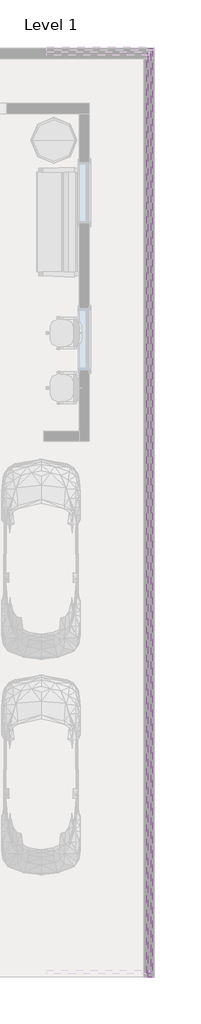
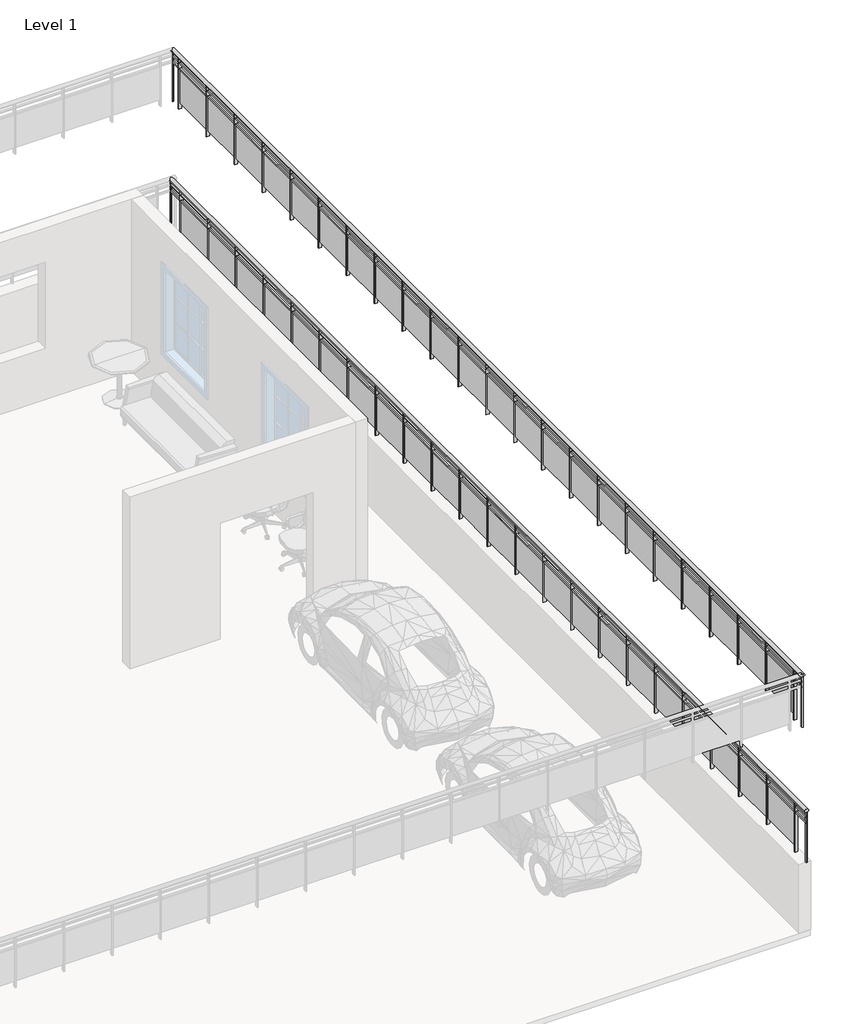
# One storey, part 4 of 6: 2 railings.
"""IFC4 building model written with IfcOpenShell, lengths in millimetres."""

from ifc_helpers import new_model, si_unit, point, frame, origin, place, context, project, spatial, polyline, ellipse_curve, trimmed, outline, extrude, element, save
from ifc_brep_helpers import plane_surface, extruded_surface, advanced_brep

model = new_model("IFC4")

# Units and contexts
model_context = context("Model", 3, world=origin())
ifc_project = project(units=[si_unit("LENGTHUNIT", "METRE", prefix="MILLI")], contexts=[model_context])

# Site, building, storey
site = spatial("IfcSite", under=ifc_project)
building = spatial("IfcBuilding", under=site)
storey = spatial("IfcBuildingStorey", under=building, Name="Level 1", Elevation=0.0)

# Railings
placement = place(None, origin())
element("IfcRailing", 1, ObjectType="Glass Panel - Bottom Fill", at=placement, inside=storey, context=model_context, shape_type="SolidModel", body=[
    advanced_brep(
    [(10487.1597674, -4490.3366944, 2133.6), (10563.3597674, -4490.3366944, 2133.6), (10487.1597674, 14000.8633056, 2133.6), (10563.3597674, 14000.8633056, 2133.6)],
    [
        (0, 1, ellipse_curve(frame((10525.2597674, -4490.3366944, 2133.6), z_axis=(0.0, -1.0, 0.0), x_axis=(1.0, 0.0, 0.0)), 38.1, 28.575)),
        (1, 0, ellipse_curve(frame((10525.2597674, -4490.3366944, 2133.6), z_axis=(0.0, -1.0, 0.0), x_axis=(1.0, 0.0, 0.0)), 38.1, 28.575)),
        (2, 3, ellipse_curve(frame((10525.2597674, 14000.8633056, 2133.6), z_axis=(0.0, 1.0, 0.0), x_axis=(1.0, 0.0, 0.0)), 38.1, 28.575)),
        (3, 2, ellipse_curve(frame((10525.2597674, 14000.8633056, 2133.6), z_axis=(0.0, 1.0, 0.0), x_axis=(1.0, 0.0, 0.0)), 38.1, 28.575)),
        (0, 2),
        (3, 1),
    ],
    [
        plane_surface(frame((10525.2597674, -4490.3366944, 2133.6), z_axis=(0.0, -1.0, 0.0), x_axis=(0.0, 0.0, 1.0))),
        plane_surface(frame((10525.2597674, 14000.8633056, 2133.6), z_axis=(0.0, 1.0, 0.0), x_axis=(0.0, 0.0, 1.0))),
        extruded_surface(trimmed(ellipse_curve(frame((10525.2597674, 14000.8633056, 2133.6), z_axis=(0.0, -1.0, 0.0), x_axis=(1.0, 0.0, 0.0)), 38.1, 28.575), [point((10487.1597674, 14000.8633056, 2133.6))], [point((10563.3597674, 14000.8633056, 2133.6))], True, "CARTESIAN"), (0.0, -18491.2, 0.0), 18491.2),
        extruded_surface(trimmed(ellipse_curve(frame((10525.2597674, 14000.8633056, 2133.6), z_axis=(0.0, -1.0, 0.0), x_axis=(1.0, 0.0, 0.0)), 38.1, 28.575), [point((10563.3597674, 14000.8633056, 2133.6))], [point((10487.1597674, 14000.8633056, 2133.6))], True, "CARTESIAN"), (0.0, -18491.2, 0.0), 18491.2),
    ],
    [
        (0, [[1, 2]]),
        (1, [[3, 4]]),
        (2, [[-1, 5, -4, 6]]),
        (3, [[-2, -6, -3, -5]]),
    ],
),
    extrude(outline(polyline([(10537.9597674, -4490.3366944), (10512.5597674, -4490.3366944), (10512.5597674, 14000.8633056), (10537.9597674, 14000.8633056), (10537.9597674, -4490.3366944)])), frame((0.0, 0.0, 2019.3), z_axis=(0.0, 0.0, 1.0), x_axis=(1.0, 0.0, 0.0)), (0.0, 0.0, 1.0), 25.4),
    extrude(outline(polyline([(10537.9597674, -4490.3366944), (10512.5597674, -4490.3366944), (10512.5597674, 14000.8633056), (10537.9597674, 14000.8633056), (10537.9597674, -4490.3366944)])), frame((0.0, 0.0, 1917.7), z_axis=(0.0, 0.0, 1.0), x_axis=(1.0, 0.0, 0.0)), (0.0, 0.0, 1.0), 25.4),
    extrude(outline(polyline([(10550.6597674, 13689.7133056), (10499.8597674, 13689.7133056), (10499.8597674, 13702.4133056), (10550.6597674, 13702.4133056), (10550.6597674, 13689.7133056)])), frame((0.0, 0.0, 1219.2), z_axis=(0.0, 0.0, 1.0), x_axis=(1.0, 0.0, 0.0)), (0.0, 0.0, 1.0), 885.6788223),
    extrude(outline(polyline([(10518.7246104, 12883.2633056), (10518.7246104, 13696.0633056), (10525.0746104, 13696.0633056), (10525.0746104, 12883.2633056), (10518.7246104, 12883.2633056)])), frame((0.0, 0.0, 1320.8), z_axis=(0.0, 0.0, 1.0), x_axis=(1.0, 0.0, 0.0)), (0.0, 0.0, 1.0), 596.9),
    extrude(outline(polyline([(10550.6597674, 12876.9133056), (10499.8597674, 12876.9133056), (10499.8597674, 12889.6133056), (10550.6597674, 12889.6133056), (10550.6597674, 12876.9133056)])), frame((0.0, 0.0, 1219.2), z_axis=(0.0, 0.0, 1.0), x_axis=(1.0, 0.0, 0.0)), (0.0, 0.0, 1.0), 885.6788223),
    extrude(outline(polyline([(10518.7246104, 12070.4633056), (10518.7246104, 12883.2633056), (10525.0746104, 12883.2633056), (10525.0746104, 12070.4633056), (10518.7246104, 12070.4633056)])), frame((0.0, 0.0, 1320.8), z_axis=(0.0, 0.0, 1.0), x_axis=(1.0, 0.0, 0.0)), (0.0, 0.0, 1.0), 596.9),
    extrude(outline(polyline([(10550.6597674, 12064.1133056), (10499.8597674, 12064.1133056), (10499.8597674, 12076.8133056), (10550.6597674, 12076.8133056), (10550.6597674, 12064.1133056)])), frame((0.0, 0.0, 1219.2), z_axis=(0.0, 0.0, 1.0), x_axis=(1.0, 0.0, 0.0)), (0.0, 0.0, 1.0), 885.6788223),
    extrude(outline(polyline([(10518.7246104, 11257.6633056), (10518.7246104, 12070.4633056), (10525.0746104, 12070.4633056), (10525.0746104, 11257.6633056), (10518.7246104, 11257.6633056)])), frame((0.0, 0.0, 1320.8), z_axis=(0.0, 0.0, 1.0), x_axis=(1.0, 0.0, 0.0)), (0.0, 0.0, 1.0), 596.9),
    extrude(outline(polyline([(10550.6597674, 11251.3133056), (10499.8597674, 11251.3133056), (10499.8597674, 11264.0133056), (10550.6597674, 11264.0133056), (10550.6597674, 11251.3133056)])), frame((0.0, 0.0, 1219.2), z_axis=(0.0, 0.0, 1.0), x_axis=(1.0, 0.0, 0.0)), (0.0, 0.0, 1.0), 885.6788223),
    extrude(outline(polyline([(10518.7246104, 10444.8633056), (10518.7246104, 11257.6633056), (10525.0746104, 11257.6633056), (10525.0746104, 10444.8633056), (10518.7246104, 10444.8633056)])), frame((0.0, 0.0, 1320.8), z_axis=(0.0, 0.0, 1.0), x_axis=(1.0, 0.0, 0.0)), (0.0, 0.0, 1.0), 596.9),
    extrude(outline(polyline([(10550.6597674, 10438.5133056), (10499.8597674, 10438.5133056), (10499.8597674, 10451.2133056), (10550.6597674, 10451.2133056), (10550.6597674, 10438.5133056)])), frame((0.0, 0.0, 1219.2), z_axis=(0.0, 0.0, 1.0), x_axis=(1.0, 0.0, 0.0)), (0.0, 0.0, 1.0), 885.6788223),
    extrude(outline(polyline([(10518.7246104, 9632.0633056), (10518.7246104, 10444.8633056), (10525.0746104, 10444.8633056), (10525.0746104, 9632.0633056), (10518.7246104, 9632.0633056)])), frame((0.0, 0.0, 1320.8), z_axis=(0.0, 0.0, 1.0), x_axis=(1.0, 0.0, 0.0)), (0.0, 0.0, 1.0), 596.9),
    extrude(outline(polyline([(10550.6597674, 9625.7133056), (10499.8597674, 9625.7133056), (10499.8597674, 9638.4133056), (10550.6597674, 9638.4133056), (10550.6597674, 9625.7133056)])), frame((0.0, 0.0, 1219.2), z_axis=(0.0, 0.0, 1.0), x_axis=(1.0, 0.0, 0.0)), (0.0, 0.0, 1.0), 885.6788223),
    extrude(outline(polyline([(10518.7246104, 8819.2633056), (10518.7246104, 9632.0633056), (10525.0746104, 9632.0633056), (10525.0746104, 8819.2633056), (10518.7246104, 8819.2633056)])), frame((0.0, 0.0, 1320.8), z_axis=(0.0, 0.0, 1.0), x_axis=(1.0, 0.0, 0.0)), (0.0, 0.0, 1.0), 596.9),
    extrude(outline(polyline([(10550.6597674, 8812.9133056), (10499.8597674, 8812.9133056), (10499.8597674, 8825.6133056), (10550.6597674, 8825.6133056), (10550.6597674, 8812.9133056)])), frame((0.0, 0.0, 1219.2), z_axis=(0.0, 0.0, 1.0), x_axis=(1.0, 0.0, 0.0)), (0.0, 0.0, 1.0), 885.6788223),
    extrude(outline(polyline([(10518.7246104, 8006.4633056), (10518.7246104, 8819.2633056), (10525.0746104, 8819.2633056), (10525.0746104, 8006.4633056), (10518.7246104, 8006.4633056)])), frame((0.0, 0.0, 1320.8), z_axis=(0.0, 0.0, 1.0), x_axis=(1.0, 0.0, 0.0)), (0.0, 0.0, 1.0), 596.9),
    extrude(outline(polyline([(10550.6597674, 8000.1133056), (10499.8597674, 8000.1133056), (10499.8597674, 8012.8133056), (10550.6597674, 8012.8133056), (10550.6597674, 8000.1133056)])), frame((0.0, 0.0, 1219.2), z_axis=(0.0, 0.0, 1.0), x_axis=(1.0, 0.0, 0.0)), (0.0, 0.0, 1.0), 885.6788223),
    extrude(outline(polyline([(10518.7246104, 7193.6633056), (10518.7246104, 8006.4633056), (10525.0746104, 8006.4633056), (10525.0746104, 7193.6633056), (10518.7246104, 7193.6633056)])), frame((0.0, 0.0, 1320.8), z_axis=(0.0, 0.0, 1.0), x_axis=(1.0, 0.0, 0.0)), (0.0, 0.0, 1.0), 596.9),
    extrude(outline(polyline([(10550.6597674, 7187.3133056), (10499.8597674, 7187.3133056), (10499.8597674, 7200.0133056), (10550.6597674, 7200.0133056), (10550.6597674, 7187.3133056)])), frame((0.0, 0.0, 1219.2), z_axis=(0.0, 0.0, 1.0), x_axis=(1.0, 0.0, 0.0)), (0.0, 0.0, 1.0), 885.6788223),
    extrude(outline(polyline([(10518.7246104, 6380.8633056), (10518.7246104, 7193.6633056), (10525.0746104, 7193.6633056), (10525.0746104, 6380.8633056), (10518.7246104, 6380.8633056)])), frame((0.0, 0.0, 1320.8), z_axis=(0.0, 0.0, 1.0), x_axis=(1.0, 0.0, 0.0)), (0.0, 0.0, 1.0), 596.9),
    extrude(outline(polyline([(10550.6597674, 6374.5133056), (10499.8597674, 6374.5133056), (10499.8597674, 6387.2133056), (10550.6597674, 6387.2133056), (10550.6597674, 6374.5133056)])), frame((0.0, 0.0, 1219.2), z_axis=(0.0, 0.0, 1.0), x_axis=(1.0, 0.0, 0.0)), (0.0, 0.0, 1.0), 885.6788223),
    extrude(outline(polyline([(10518.7246104, 5568.0633056), (10518.7246104, 6380.8633056), (10525.0746104, 6380.8633056), (10525.0746104, 5568.0633056), (10518.7246104, 5568.0633056)])), frame((0.0, 0.0, 1320.8), z_axis=(0.0, 0.0, 1.0), x_axis=(1.0, 0.0, 0.0)), (0.0, 0.0, 1.0), 596.9),
    extrude(outline(polyline([(10550.6597674, 5561.7133056), (10499.8597674, 5561.7133056), (10499.8597674, 5574.4133056), (10550.6597674, 5574.4133056), (10550.6597674, 5561.7133056)])), frame((0.0, 0.0, 1219.2), z_axis=(0.0, 0.0, 1.0), x_axis=(1.0, 0.0, 0.0)), (0.0, 0.0, 1.0), 885.6788223),
    extrude(outline(polyline([(10518.7246104, 4755.2633056), (10518.7246104, 5568.0633056), (10525.0746104, 5568.0633056), (10525.0746104, 4755.2633056), (10518.7246104, 4755.2633056)])), frame((0.0, 0.0, 1320.8), z_axis=(0.0, 0.0, 1.0), x_axis=(1.0, 0.0, 0.0)), (0.0, 0.0, 1.0), 596.9),
    extrude(outline(polyline([(10550.6597674, 4748.9133056), (10499.8597674, 4748.9133056), (10499.8597674, 4761.6133056), (10550.6597674, 4761.6133056), (10550.6597674, 4748.9133056)])), frame((0.0, 0.0, 1219.2), z_axis=(0.0, 0.0, 1.0), x_axis=(1.0, 0.0, 0.0)), (0.0, 0.0, 1.0), 885.6788223),
    extrude(outline(polyline([(10518.7246104, 3942.4633056), (10518.7246104, 4755.2633056), (10525.0746104, 4755.2633056), (10525.0746104, 3942.4633056), (10518.7246104, 3942.4633056)])), frame((0.0, 0.0, 1320.8), z_axis=(0.0, 0.0, 1.0), x_axis=(1.0, 0.0, 0.0)), (0.0, 0.0, 1.0), 596.9),
    extrude(outline(polyline([(10550.6597674, 3936.1133056), (10499.8597674, 3936.1133056), (10499.8597674, 3948.8133056), (10550.6597674, 3948.8133056), (10550.6597674, 3936.1133056)])), frame((0.0, 0.0, 1219.2), z_axis=(0.0, 0.0, 1.0), x_axis=(1.0, 0.0, 0.0)), (0.0, 0.0, 1.0), 885.6788223),
    extrude(outline(polyline([(10518.7246104, 3129.6633056), (10518.7246104, 3942.4633056), (10525.0746104, 3942.4633056), (10525.0746104, 3129.6633056), (10518.7246104, 3129.6633056)])), frame((0.0, 0.0, 1320.8), z_axis=(0.0, 0.0, 1.0), x_axis=(1.0, 0.0, 0.0)), (0.0, 0.0, 1.0), 596.9),
    extrude(outline(polyline([(10550.6597674, 3123.3133056), (10499.8597674, 3123.3133056), (10499.8597674, 3136.0133056), (10550.6597674, 3136.0133056), (10550.6597674, 3123.3133056)])), frame((0.0, 0.0, 1219.2), z_axis=(0.0, 0.0, 1.0), x_axis=(1.0, 0.0, 0.0)), (0.0, 0.0, 1.0), 885.6788223),
    extrude(outline(polyline([(10518.7246104, 2316.8633056), (10518.7246104, 3129.6633056), (10525.0746104, 3129.6633056), (10525.0746104, 2316.8633056), (10518.7246104, 2316.8633056)])), frame((0.0, 0.0, 1320.8), z_axis=(0.0, 0.0, 1.0), x_axis=(1.0, 0.0, 0.0)), (0.0, 0.0, 1.0), 596.9),
    extrude(outline(polyline([(10550.6597674, 2310.5133056), (10499.8597674, 2310.5133056), (10499.8597674, 2323.2133056), (10550.6597674, 2323.2133056), (10550.6597674, 2310.5133056)])), frame((0.0, 0.0, 1219.2), z_axis=(0.0, 0.0, 1.0), x_axis=(1.0, 0.0, 0.0)), (0.0, 0.0, 1.0), 885.6788223),
    extrude(outline(polyline([(10518.7246104, 1504.0633056), (10518.7246104, 2316.8633056), (10525.0746104, 2316.8633056), (10525.0746104, 1504.0633056), (10518.7246104, 1504.0633056)])), frame((0.0, 0.0, 1320.8), z_axis=(0.0, 0.0, 1.0), x_axis=(1.0, 0.0, 0.0)), (0.0, 0.0, 1.0), 596.9),
    extrude(outline(polyline([(10550.6597674, 1497.7133056), (10499.8597674, 1497.7133056), (10499.8597674, 1510.4133056), (10550.6597674, 1510.4133056), (10550.6597674, 1497.7133056)])), frame((0.0, 0.0, 1219.2), z_axis=(0.0, 0.0, 1.0), x_axis=(1.0, 0.0, 0.0)), (0.0, 0.0, 1.0), 885.6788223),
    extrude(outline(polyline([(10518.7246104, 691.2633056), (10518.7246104, 1504.0633056), (10525.0746104, 1504.0633056), (10525.0746104, 691.2633056), (10518.7246104, 691.2633056)])), frame((0.0, 0.0, 1320.8), z_axis=(0.0, 0.0, 1.0), x_axis=(1.0, 0.0, 0.0)), (0.0, 0.0, 1.0), 596.9),
    extrude(outline(polyline([(10550.6597674, 684.9133056), (10499.8597674, 684.9133056), (10499.8597674, 697.6133056), (10550.6597674, 697.6133056), (10550.6597674, 684.9133056)])), frame((0.0, 0.0, 1219.2), z_axis=(0.0, 0.0, 1.0), x_axis=(1.0, 0.0, 0.0)), (0.0, 0.0, 1.0), 885.6788223),
    extrude(outline(polyline([(10518.7246104, -121.5366944), (10518.7246104, 691.2633056), (10525.0746104, 691.2633056), (10525.0746104, -121.5366944), (10518.7246104, -121.5366944)])), frame((0.0, 0.0, 1320.8), z_axis=(0.0, 0.0, 1.0), x_axis=(1.0, 0.0, 0.0)), (0.0, 0.0, 1.0), 596.9),
    extrude(outline(polyline([(10550.6597674, -127.8866944), (10499.8597674, -127.8866944), (10499.8597674, -115.1866944), (10550.6597674, -115.1866944), (10550.6597674, -127.8866944)])), frame((0.0, 0.0, 1219.2), z_axis=(0.0, 0.0, 1.0), x_axis=(1.0, 0.0, 0.0)), (0.0, 0.0, 1.0), 885.6788223),
    extrude(outline(polyline([(10518.7246104, -934.3366944), (10518.7246104, -121.5366944), (10525.0746104, -121.5366944), (10525.0746104, -934.3366944), (10518.7246104, -934.3366944)])), frame((0.0, 0.0, 1320.8), z_axis=(0.0, 0.0, 1.0), x_axis=(1.0, 0.0, 0.0)), (0.0, 0.0, 1.0), 596.9),
    extrude(outline(polyline([(10550.6597674, -940.6866944), (10499.8597674, -940.6866944), (10499.8597674, -927.9866944), (10550.6597674, -927.9866944), (10550.6597674, -940.6866944)])), frame((0.0, 0.0, 1219.2), z_axis=(0.0, 0.0, 1.0), x_axis=(1.0, 0.0, 0.0)), (0.0, 0.0, 1.0), 885.6788223),
    extrude(outline(polyline([(10518.7246104, -1747.1366944), (10518.7246104, -934.3366944), (10525.0746104, -934.3366944), (10525.0746104, -1747.1366944), (10518.7246104, -1747.1366944)])), frame((0.0, 0.0, 1320.8), z_axis=(0.0, 0.0, 1.0), x_axis=(1.0, 0.0, 0.0)), (0.0, 0.0, 1.0), 596.9),
    extrude(outline(polyline([(10550.6597674, -1753.4866944), (10499.8597674, -1753.4866944), (10499.8597674, -1740.7866944), (10550.6597674, -1740.7866944), (10550.6597674, -1753.4866944)])), frame((0.0, 0.0, 1219.2), z_axis=(0.0, 0.0, 1.0), x_axis=(1.0, 0.0, 0.0)), (0.0, 0.0, 1.0), 885.6788223),
    extrude(outline(polyline([(10518.7246104, -2559.9366944), (10518.7246104, -1747.1366944), (10525.0746104, -1747.1366944), (10525.0746104, -2559.9366944), (10518.7246104, -2559.9366944)])), frame((0.0, 0.0, 1320.8), z_axis=(0.0, 0.0, 1.0), x_axis=(1.0, 0.0, 0.0)), (0.0, 0.0, 1.0), 596.9),
    extrude(outline(polyline([(10550.6597674, -2566.2866944), (10499.8597674, -2566.2866944), (10499.8597674, -2553.5866944), (10550.6597674, -2553.5866944), (10550.6597674, -2566.2866944)])), frame((0.0, 0.0, 1219.2), z_axis=(0.0, 0.0, 1.0), x_axis=(1.0, 0.0, 0.0)), (0.0, 0.0, 1.0), 885.6788223),
    extrude(outline(polyline([(10518.7246104, -3372.7366944), (10518.7246104, -2559.9366944), (10525.0746104, -2559.9366944), (10525.0746104, -3372.7366944), (10518.7246104, -3372.7366944)])), frame((0.0, 0.0, 1320.8), z_axis=(0.0, 0.0, 1.0), x_axis=(1.0, 0.0, 0.0)), (0.0, 0.0, 1.0), 596.9),
    extrude(outline(polyline([(10550.6597674, -3379.0866944), (10499.8597674, -3379.0866944), (10499.8597674, -3366.3866944), (10550.6597674, -3366.3866944), (10550.6597674, -3379.0866944)])), frame((0.0, 0.0, 1219.2), z_axis=(0.0, 0.0, 1.0), x_axis=(1.0, 0.0, 0.0)), (0.0, 0.0, 1.0), 885.6788223),
    extrude(outline(polyline([(10518.7246104, -4185.5366944), (10518.7246104, -3372.7366944), (10525.0746104, -3372.7366944), (10525.0746104, -4185.5366944), (10518.7246104, -4185.5366944)])), frame((0.0, 0.0, 1320.8), z_axis=(0.0, 0.0, 1.0), x_axis=(1.0, 0.0, 0.0)), (0.0, 0.0, 1.0), 596.9),
    extrude(outline(polyline([(10550.6597674, -4191.8866944), (10499.8597674, -4191.8866944), (10499.8597674, -4179.1866944), (10550.6597674, -4179.1866944), (10550.6597674, -4191.8866944)])), frame((0.0, 0.0, 1219.2), z_axis=(0.0, 0.0, 1.0), x_axis=(1.0, 0.0, 0.0)), (0.0, 0.0, 1.0), 885.6788223),
    extrude(outline(polyline([(10534.7847674, 13988.1633056), (10515.7347674, 13988.1633056), (10515.7347674, 14007.2133056), (10534.7847674, 14007.2133056), (10534.7847674, 13988.1633056)])), frame((0.0, 0.0, 1219.2), z_axis=(0.0, 0.0, 1.0), x_axis=(1.0, 0.0, 0.0)), (0.0, 0.0, 1.0), 885.6788223),
    extrude(outline(polyline([(10534.7847674, -4496.6866944), (10515.7347674, -4496.6866944), (10515.7347674, -4477.6366944), (10534.7847674, -4477.6366944), (10534.7847674, -4496.6866944)])), frame((0.0, 0.0, 1219.2), z_axis=(0.0, 0.0, 1.0), x_axis=(1.0, 0.0, 0.0)), (0.0, 0.0, 1.0), 885.6788223),
])
element("IfcRailing", 2, ObjectType="Glass Panel - Bottom Fill", at=placement, inside=storey, context=model_context, shape_type="SolidModel", body=[
    advanced_brep(
    [(10461.7597674, -4414.1366944, 4495.8), (10537.9597674, -4414.1366944, 4495.8), (10461.7597674, 13899.2633056, 4495.8), (10537.9597674, 13899.2633056, 4495.8)],
    [
        (0, 1, ellipse_curve(frame((10499.8597674, -4414.1366944, 4495.8), z_axis=(0.0, -1.0, 0.0), x_axis=(1.0, 0.0, 0.0)), 38.1, 28.575)),
        (1, 0, ellipse_curve(frame((10499.8597674, -4414.1366944, 4495.8), z_axis=(0.0, -1.0, 0.0), x_axis=(1.0, 0.0, 0.0)), 38.1, 28.575)),
        (2, 3, ellipse_curve(frame((10499.8597674, 13899.2633056, 4495.8), z_axis=(0.0, 1.0, 0.0), x_axis=(1.0, 0.0, 0.0)), 38.1, 28.575)),
        (3, 2, ellipse_curve(frame((10499.8597674, 13899.2633056, 4495.8), z_axis=(0.0, 1.0, 0.0), x_axis=(1.0, 0.0, 0.0)), 38.1, 28.575)),
        (0, 2),
        (3, 1),
    ],
    [
        plane_surface(frame((10499.8597674, -4414.1366944, 4495.8), z_axis=(0.0, -1.0, 0.0), x_axis=(0.0, 0.0, 1.0))),
        plane_surface(frame((10499.8597674, 13899.2633056, 4495.8), z_axis=(0.0, 1.0, 0.0), x_axis=(0.0, 0.0, 1.0))),
        extruded_surface(trimmed(ellipse_curve(frame((10499.8597674, 13899.2633056, 4495.8), z_axis=(0.0, -1.0, 0.0), x_axis=(1.0, 0.0, 0.0)), 38.1, 28.575), [point((10461.7597674, 13899.2633056, 4495.8))], [point((10537.9597674, 13899.2633056, 4495.8))], True, "CARTESIAN"), (0.0, -18313.4, 0.0), 18313.4),
        extruded_surface(trimmed(ellipse_curve(frame((10499.8597674, 13899.2633056, 4495.8), z_axis=(0.0, -1.0, 0.0), x_axis=(1.0, 0.0, 0.0)), 38.1, 28.575), [point((10537.9597674, 13899.2633056, 4495.8))], [point((10461.7597674, 13899.2633056, 4495.8))], True, "CARTESIAN"), (0.0, -18313.4, 0.0), 18313.4),
    ],
    [
        (0, [[1, 2]]),
        (1, [[3, 4]]),
        (2, [[-1, 5, -4, 6]]),
        (3, [[-2, -6, -3, -5]]),
    ],
),
    extrude(outline(polyline([(10512.5597674, -4414.1366944), (10487.1597674, -4414.1366944), (10487.1597674, 13899.2633056), (10512.5597674, 13899.2633056), (10512.5597674, -4414.1366944)])), frame((0.0, 0.0, 4381.5), z_axis=(0.0, 0.0, 1.0), x_axis=(1.0, 0.0, 0.0)), (0.0, 0.0, 1.0), 25.4),
    extrude(outline(polyline([(10512.5597674, -4414.1366944), (10487.1597674, -4414.1366944), (10487.1597674, 13899.2633056), (10512.5597674, 13899.2633056), (10512.5597674, -4414.1366944)])), frame((0.0, 0.0, 4279.9), z_axis=(0.0, 0.0, 1.0), x_axis=(1.0, 0.0, 0.0)), (0.0, 0.0, 1.0), 25.4),
    extrude(outline(polyline([(10525.2597674, 13677.0133056), (10474.4597674, 13677.0133056), (10474.4597674, 13689.7133056), (10525.2597674, 13689.7133056), (10525.2597674, 13677.0133056)])), frame((0.0, 0.0, 3581.4), z_axis=(0.0, 0.0, 1.0), x_axis=(1.0, 0.0, 0.0)), (0.0, 0.0, 1.0), 885.6788223),
    extrude(outline(polyline([(10493.3246104, 12870.5633056), (10493.3246104, 13683.3633056), (10499.6746104, 13683.3633056), (10499.6746104, 12870.5633056), (10493.3246104, 12870.5633056)])), frame((0.0, 0.0, 3683.0), z_axis=(0.0, 0.0, 1.0), x_axis=(1.0, 0.0, 0.0)), (0.0, 0.0, 1.0), 596.9),
    extrude(outline(polyline([(10525.2597674, 12864.2133056), (10474.4597674, 12864.2133056), (10474.4597674, 12876.9133056), (10525.2597674, 12876.9133056), (10525.2597674, 12864.2133056)])), frame((0.0, 0.0, 3581.4), z_axis=(0.0, 0.0, 1.0), x_axis=(1.0, 0.0, 0.0)), (0.0, 0.0, 1.0), 885.6788223),
    extrude(outline(polyline([(10493.3246104, 12057.7633056), (10493.3246104, 12870.5633056), (10499.6746104, 12870.5633056), (10499.6746104, 12057.7633056), (10493.3246104, 12057.7633056)])), frame((0.0, 0.0, 3683.0), z_axis=(0.0, 0.0, 1.0), x_axis=(1.0, 0.0, 0.0)), (0.0, 0.0, 1.0), 596.9),
    extrude(outline(polyline([(10525.2597674, 12051.4133056), (10474.4597674, 12051.4133056), (10474.4597674, 12064.1133056), (10525.2597674, 12064.1133056), (10525.2597674, 12051.4133056)])), frame((0.0, 0.0, 3581.4), z_axis=(0.0, 0.0, 1.0), x_axis=(1.0, 0.0, 0.0)), (0.0, 0.0, 1.0), 885.6788223),
    extrude(outline(polyline([(10493.3246104, 11244.9633056), (10493.3246104, 12057.7633056), (10499.6746104, 12057.7633056), (10499.6746104, 11244.9633056), (10493.3246104, 11244.9633056)])), frame((0.0, 0.0, 3683.0), z_axis=(0.0, 0.0, 1.0), x_axis=(1.0, 0.0, 0.0)), (0.0, 0.0, 1.0), 596.9),
    extrude(outline(polyline([(10525.2597674, 11238.6133056), (10474.4597674, 11238.6133056), (10474.4597674, 11251.3133056), (10525.2597674, 11251.3133056), (10525.2597674, 11238.6133056)])), frame((0.0, 0.0, 3581.4), z_axis=(0.0, 0.0, 1.0), x_axis=(1.0, 0.0, 0.0)), (0.0, 0.0, 1.0), 885.6788223),
    extrude(outline(polyline([(10493.3246104, 10432.1633056), (10493.3246104, 11244.9633056), (10499.6746104, 11244.9633056), (10499.6746104, 10432.1633056), (10493.3246104, 10432.1633056)])), frame((0.0, 0.0, 3683.0), z_axis=(0.0, 0.0, 1.0), x_axis=(1.0, 0.0, 0.0)), (0.0, 0.0, 1.0), 596.9),
    extrude(outline(polyline([(10525.2597674, 10425.8133056), (10474.4597674, 10425.8133056), (10474.4597674, 10438.5133056), (10525.2597674, 10438.5133056), (10525.2597674, 10425.8133056)])), frame((0.0, 0.0, 3581.4), z_axis=(0.0, 0.0, 1.0), x_axis=(1.0, 0.0, 0.0)), (0.0, 0.0, 1.0), 885.6788223),
    extrude(outline(polyline([(10493.3246104, 9619.3633056), (10493.3246104, 10432.1633056), (10499.6746104, 10432.1633056), (10499.6746104, 9619.3633056), (10493.3246104, 9619.3633056)])), frame((0.0, 0.0, 3683.0), z_axis=(0.0, 0.0, 1.0), x_axis=(1.0, 0.0, 0.0)), (0.0, 0.0, 1.0), 596.9),
    extrude(outline(polyline([(10525.2597674, 9613.0133056), (10474.4597674, 9613.0133056), (10474.4597674, 9625.7133056), (10525.2597674, 9625.7133056), (10525.2597674, 9613.0133056)])), frame((0.0, 0.0, 3581.4), z_axis=(0.0, 0.0, 1.0), x_axis=(1.0, 0.0, 0.0)), (0.0, 0.0, 1.0), 885.6788223),
    extrude(outline(polyline([(10493.3246104, 8806.5633056), (10493.3246104, 9619.3633056), (10499.6746104, 9619.3633056), (10499.6746104, 8806.5633056), (10493.3246104, 8806.5633056)])), frame((0.0, 0.0, 3683.0), z_axis=(0.0, 0.0, 1.0), x_axis=(1.0, 0.0, 0.0)), (0.0, 0.0, 1.0), 596.9),
    extrude(outline(polyline([(10525.2597674, 8800.2133056), (10474.4597674, 8800.2133056), (10474.4597674, 8812.9133056), (10525.2597674, 8812.9133056), (10525.2597674, 8800.2133056)])), frame((0.0, 0.0, 3581.4), z_axis=(0.0, 0.0, 1.0), x_axis=(1.0, 0.0, 0.0)), (0.0, 0.0, 1.0), 885.6788223),
    extrude(outline(polyline([(10493.3246104, 7993.7633056), (10493.3246104, 8806.5633056), (10499.6746104, 8806.5633056), (10499.6746104, 7993.7633056), (10493.3246104, 7993.7633056)])), frame((0.0, 0.0, 3683.0), z_axis=(0.0, 0.0, 1.0), x_axis=(1.0, 0.0, 0.0)), (0.0, 0.0, 1.0), 596.9),
    extrude(outline(polyline([(10525.2597674, 7987.4133056), (10474.4597674, 7987.4133056), (10474.4597674, 8000.1133056), (10525.2597674, 8000.1133056), (10525.2597674, 7987.4133056)])), frame((0.0, 0.0, 3581.4), z_axis=(0.0, 0.0, 1.0), x_axis=(1.0, 0.0, 0.0)), (0.0, 0.0, 1.0), 885.6788223),
    extrude(outline(polyline([(10493.3246104, 7180.9633056), (10493.3246104, 7993.7633056), (10499.6746104, 7993.7633056), (10499.6746104, 7180.9633056), (10493.3246104, 7180.9633056)])), frame((0.0, 0.0, 3683.0), z_axis=(0.0, 0.0, 1.0), x_axis=(1.0, 0.0, 0.0)), (0.0, 0.0, 1.0), 596.9),
    extrude(outline(polyline([(10525.2597674, 7174.6133056), (10474.4597674, 7174.6133056), (10474.4597674, 7187.3133056), (10525.2597674, 7187.3133056), (10525.2597674, 7174.6133056)])), frame((0.0, 0.0, 3581.4), z_axis=(0.0, 0.0, 1.0), x_axis=(1.0, 0.0, 0.0)), (0.0, 0.0, 1.0), 885.6788223),
    extrude(outline(polyline([(10493.3246104, 6368.1633056), (10493.3246104, 7180.9633056), (10499.6746104, 7180.9633056), (10499.6746104, 6368.1633056), (10493.3246104, 6368.1633056)])), frame((0.0, 0.0, 3683.0), z_axis=(0.0, 0.0, 1.0), x_axis=(1.0, 0.0, 0.0)), (0.0, 0.0, 1.0), 596.9),
    extrude(outline(polyline([(10525.2597674, 6361.8133056), (10474.4597674, 6361.8133056), (10474.4597674, 6374.5133056), (10525.2597674, 6374.5133056), (10525.2597674, 6361.8133056)])), frame((0.0, 0.0, 3581.4), z_axis=(0.0, 0.0, 1.0), x_axis=(1.0, 0.0, 0.0)), (0.0, 0.0, 1.0), 885.6788223),
    extrude(outline(polyline([(10493.3246104, 5555.3633056), (10493.3246104, 6368.1633056), (10499.6746104, 6368.1633056), (10499.6746104, 5555.3633056), (10493.3246104, 5555.3633056)])), frame((0.0, 0.0, 3683.0), z_axis=(0.0, 0.0, 1.0), x_axis=(1.0, 0.0, 0.0)), (0.0, 0.0, 1.0), 596.9),
    extrude(outline(polyline([(10525.2597674, 5549.0133056), (10474.4597674, 5549.0133056), (10474.4597674, 5561.7133056), (10525.2597674, 5561.7133056), (10525.2597674, 5549.0133056)])), frame((0.0, 0.0, 3581.4), z_axis=(0.0, 0.0, 1.0), x_axis=(1.0, 0.0, 0.0)), (0.0, 0.0, 1.0), 885.6788223),
    extrude(outline(polyline([(10493.3246104, 4742.5633056), (10493.3246104, 5555.3633056), (10499.6746104, 5555.3633056), (10499.6746104, 4742.5633056), (10493.3246104, 4742.5633056)])), frame((0.0, 0.0, 3683.0), z_axis=(0.0, 0.0, 1.0), x_axis=(1.0, 0.0, 0.0)), (0.0, 0.0, 1.0), 596.9),
    extrude(outline(polyline([(10525.2597674, 4736.2133056), (10474.4597674, 4736.2133056), (10474.4597674, 4748.9133056), (10525.2597674, 4748.9133056), (10525.2597674, 4736.2133056)])), frame((0.0, 0.0, 3581.4), z_axis=(0.0, 0.0, 1.0), x_axis=(1.0, 0.0, 0.0)), (0.0, 0.0, 1.0), 885.6788223),
    extrude(outline(polyline([(10493.3246104, 3929.7633056), (10493.3246104, 4742.5633056), (10499.6746104, 4742.5633056), (10499.6746104, 3929.7633056), (10493.3246104, 3929.7633056)])), frame((0.0, 0.0, 3683.0), z_axis=(0.0, 0.0, 1.0), x_axis=(1.0, 0.0, 0.0)), (0.0, 0.0, 1.0), 596.9),
    extrude(outline(polyline([(10525.2597674, 3923.4133056), (10474.4597674, 3923.4133056), (10474.4597674, 3936.1133056), (10525.2597674, 3936.1133056), (10525.2597674, 3923.4133056)])), frame((0.0, 0.0, 3581.4), z_axis=(0.0, 0.0, 1.0), x_axis=(1.0, 0.0, 0.0)), (0.0, 0.0, 1.0), 885.6788223),
    extrude(outline(polyline([(10493.3246104, 3116.9633056), (10493.3246104, 3929.7633056), (10499.6746104, 3929.7633056), (10499.6746104, 3116.9633056), (10493.3246104, 3116.9633056)])), frame((0.0, 0.0, 3683.0), z_axis=(0.0, 0.0, 1.0), x_axis=(1.0, 0.0, 0.0)), (0.0, 0.0, 1.0), 596.9),
    extrude(outline(polyline([(10525.2597674, 3110.6133056), (10474.4597674, 3110.6133056), (10474.4597674, 3123.3133056), (10525.2597674, 3123.3133056), (10525.2597674, 3110.6133056)])), frame((0.0, 0.0, 3581.4), z_axis=(0.0, 0.0, 1.0), x_axis=(1.0, 0.0, 0.0)), (0.0, 0.0, 1.0), 885.6788223),
    extrude(outline(polyline([(10493.3246104, 2304.1633056), (10493.3246104, 3116.9633056), (10499.6746104, 3116.9633056), (10499.6746104, 2304.1633056), (10493.3246104, 2304.1633056)])), frame((0.0, 0.0, 3683.0), z_axis=(0.0, 0.0, 1.0), x_axis=(1.0, 0.0, 0.0)), (0.0, 0.0, 1.0), 596.9),
    extrude(outline(polyline([(10525.2597674, 2297.8133056), (10474.4597674, 2297.8133056), (10474.4597674, 2310.5133056), (10525.2597674, 2310.5133056), (10525.2597674, 2297.8133056)])), frame((0.0, 0.0, 3581.4), z_axis=(0.0, 0.0, 1.0), x_axis=(1.0, 0.0, 0.0)), (0.0, 0.0, 1.0), 885.6788223),
    extrude(outline(polyline([(10493.3246104, 1491.3633056), (10493.3246104, 2304.1633056), (10499.6746104, 2304.1633056), (10499.6746104, 1491.3633056), (10493.3246104, 1491.3633056)])), frame((0.0, 0.0, 3683.0), z_axis=(0.0, 0.0, 1.0), x_axis=(1.0, 0.0, 0.0)), (0.0, 0.0, 1.0), 596.9),
    extrude(outline(polyline([(10525.2597674, 1485.0133056), (10474.4597674, 1485.0133056), (10474.4597674, 1497.7133056), (10525.2597674, 1497.7133056), (10525.2597674, 1485.0133056)])), frame((0.0, 0.0, 3581.4), z_axis=(0.0, 0.0, 1.0), x_axis=(1.0, 0.0, 0.0)), (0.0, 0.0, 1.0), 885.6788223),
    extrude(outline(polyline([(10493.3246104, 678.5633056), (10493.3246104, 1491.3633056), (10499.6746104, 1491.3633056), (10499.6746104, 678.5633056), (10493.3246104, 678.5633056)])), frame((0.0, 0.0, 3683.0), z_axis=(0.0, 0.0, 1.0), x_axis=(1.0, 0.0, 0.0)), (0.0, 0.0, 1.0), 596.9),
    extrude(outline(polyline([(10525.2597674, 672.2133056), (10474.4597674, 672.2133056), (10474.4597674, 684.9133056), (10525.2597674, 684.9133056), (10525.2597674, 672.2133056)])), frame((0.0, 0.0, 3581.4), z_axis=(0.0, 0.0, 1.0), x_axis=(1.0, 0.0, 0.0)), (0.0, 0.0, 1.0), 885.6788223),
    extrude(outline(polyline([(10493.3246104, -134.2366944), (10493.3246104, 678.5633056), (10499.6746104, 678.5633056), (10499.6746104, -134.2366944), (10493.3246104, -134.2366944)])), frame((0.0, 0.0, 3683.0), z_axis=(0.0, 0.0, 1.0), x_axis=(1.0, 0.0, 0.0)), (0.0, 0.0, 1.0), 596.9),
    extrude(outline(polyline([(10525.2597674, -140.5866944), (10474.4597674, -140.5866944), (10474.4597674, -127.8866944), (10525.2597674, -127.8866944), (10525.2597674, -140.5866944)])), frame((0.0, 0.0, 3581.4), z_axis=(0.0, 0.0, 1.0), x_axis=(1.0, 0.0, 0.0)), (0.0, 0.0, 1.0), 885.6788223),
    extrude(outline(polyline([(10493.3246104, -947.0366944), (10493.3246104, -134.2366944), (10499.6746104, -134.2366944), (10499.6746104, -947.0366944), (10493.3246104, -947.0366944)])), frame((0.0, 0.0, 3683.0), z_axis=(0.0, 0.0, 1.0), x_axis=(1.0, 0.0, 0.0)), (0.0, 0.0, 1.0), 596.9),
    extrude(outline(polyline([(10525.2597674, -953.3866944), (10474.4597674, -953.3866944), (10474.4597674, -940.6866944), (10525.2597674, -940.6866944), (10525.2597674, -953.3866944)])), frame((0.0, 0.0, 3581.4), z_axis=(0.0, 0.0, 1.0), x_axis=(1.0, 0.0, 0.0)), (0.0, 0.0, 1.0), 885.6788223),
    extrude(outline(polyline([(10493.3246104, -1759.8366944), (10493.3246104, -947.0366944), (10499.6746104, -947.0366944), (10499.6746104, -1759.8366944), (10493.3246104, -1759.8366944)])), frame((0.0, 0.0, 3683.0), z_axis=(0.0, 0.0, 1.0), x_axis=(1.0, 0.0, 0.0)), (0.0, 0.0, 1.0), 596.9),
    extrude(outline(polyline([(10525.2597674, -1766.1866944), (10474.4597674, -1766.1866944), (10474.4597674, -1753.4866944), (10525.2597674, -1753.4866944), (10525.2597674, -1766.1866944)])), frame((0.0, 0.0, 3581.4), z_axis=(0.0, 0.0, 1.0), x_axis=(1.0, 0.0, 0.0)), (0.0, 0.0, 1.0), 885.6788223),
    extrude(outline(polyline([(10493.3246104, -2572.6366944), (10493.3246104, -1759.8366944), (10499.6746104, -1759.8366944), (10499.6746104, -2572.6366944), (10493.3246104, -2572.6366944)])), frame((0.0, 0.0, 3683.0), z_axis=(0.0, 0.0, 1.0), x_axis=(1.0, 0.0, 0.0)), (0.0, 0.0, 1.0), 596.9),
    extrude(outline(polyline([(10525.2597674, -2578.9866944), (10474.4597674, -2578.9866944), (10474.4597674, -2566.2866944), (10525.2597674, -2566.2866944), (10525.2597674, -2578.9866944)])), frame((0.0, 0.0, 3581.4), z_axis=(0.0, 0.0, 1.0), x_axis=(1.0, 0.0, 0.0)), (0.0, 0.0, 1.0), 885.6788223),
    extrude(outline(polyline([(10493.3246104, -3385.4366944), (10493.3246104, -2572.6366944), (10499.6746104, -2572.6366944), (10499.6746104, -3385.4366944), (10493.3246104, -3385.4366944)])), frame((0.0, 0.0, 3683.0), z_axis=(0.0, 0.0, 1.0), x_axis=(1.0, 0.0, 0.0)), (0.0, 0.0, 1.0), 596.9),
    extrude(outline(polyline([(10525.2597674, -3391.7866944), (10474.4597674, -3391.7866944), (10474.4597674, -3379.0866944), (10525.2597674, -3379.0866944), (10525.2597674, -3391.7866944)])), frame((0.0, 0.0, 3581.4), z_axis=(0.0, 0.0, 1.0), x_axis=(1.0, 0.0, 0.0)), (0.0, 0.0, 1.0), 885.6788223),
    extrude(outline(polyline([(10493.3246104, -4198.2366944), (10493.3246104, -3385.4366944), (10499.6746104, -3385.4366944), (10499.6746104, -4198.2366944), (10493.3246104, -4198.2366944)])), frame((0.0, 0.0, 3683.0), z_axis=(0.0, 0.0, 1.0), x_axis=(1.0, 0.0, 0.0)), (0.0, 0.0, 1.0), 596.9),
    extrude(outline(polyline([(10525.2597674, -4204.5866944), (10474.4597674, -4204.5866944), (10474.4597674, -4191.8866944), (10525.2597674, -4191.8866944), (10525.2597674, -4204.5866944)])), frame((0.0, 0.0, 3581.4), z_axis=(0.0, 0.0, 1.0), x_axis=(1.0, 0.0, 0.0)), (0.0, 0.0, 1.0), 885.6788223),
    extrude(outline(polyline([(10509.3847674, 13886.5633056), (10490.3347674, 13886.5633056), (10490.3347674, 13905.6133056), (10509.3847674, 13905.6133056), (10509.3847674, 13886.5633056)])), frame((0.0, 0.0, 3581.4), z_axis=(0.0, 0.0, 1.0), x_axis=(1.0, 0.0, 0.0)), (0.0, 0.0, 1.0), 885.6788223),
    extrude(outline(polyline([(10509.3847674, -4420.4866944), (10490.3347674, -4420.4866944), (10490.3347674, -4401.4366944), (10509.3847674, -4401.4366944), (10509.3847674, -4420.4866944)])), frame((0.0, 0.0, 3581.4), z_axis=(0.0, 0.0, 1.0), x_axis=(1.0, 0.0, 0.0)), (0.0, 0.0, 1.0), 885.6788223),
])

save(model, "model.ifc")

# Revit data of these elements
# Type "Glass Panel - Bottom Fill"
#   Assembly Code = "C2010400"
#   built-in parameter 1008612 = 0.0416667 (stored number, unit not read)
#   built-in parameter 1008611 = 0.0416667 (stored number, unit not read)
#   built-in parameter 1008609 = 0.333333 (stored number, unit not read)
#   built-in parameter 1008604 = 0.166667 (stored number, unit not read)
#   built-in parameter 1008603 = 0.166667 (stored number, unit not read)
#   Railing Height = 3' - 0"
#   built-in parameter 1008630 = 2
#   built-in parameter 1008610 = 2
#   built-in parameter 1008618 = Baluster - Square : 3/4"
# Element 1 (IfcRailing, "Glass Panel - Bottom Fill")
#   built-in parameter 1008621 = 4 (stored number, unit not read)
#   Phase Created = New Construction
#   Materials on its faces: "Glass"
# Element 2 (IfcRailing, "Glass Panel - Bottom Fill")
#   built-in parameter 1008621 = 11.75 (stored number, unit not read)
#   Phase Created = New Construction
#   Materials on its faces: "Glass"
# Materials
#   "Glass": class "Glass", colour RGB 0 128 192, transparency 0.75, Description = "Soda Lime Glass", Cost = 0
